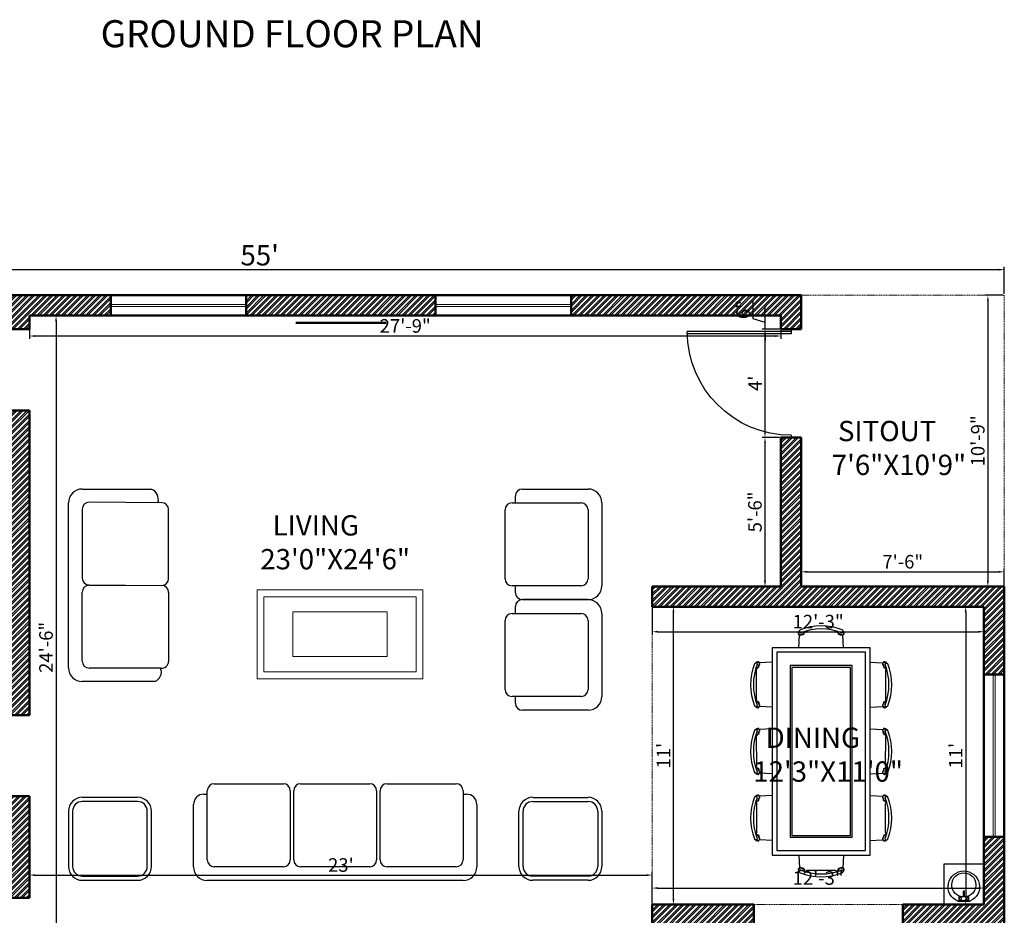
# Model space of a CAD drawing. Units: inches. Extents: x 3590 to 5167, y 65 to 1917.
# Tile 6 of 100: x 3869 to 4306, y 314 to 711. Entities that reach past the tile are written whole.
import ezdxf

# ---------------------------------------------------------------- set-up
doc = ezdxf.new("R2010")
doc.units = ezdxf.units.IN
doc.linetypes.add('DASHED', pattern=[0.75, 0.5, -0.25])
for name, color, linetype, lineweight in [('A-ANNO-DIMS', 2, 'Continuous', 18), ('A-ANNO-TEXT', 7, 'Continuous', 25), ('A-AREA-IDEN', 7, 'Continuous', 18), ('A-DOOR', 3, 'Continuous', 25), ('A-FLOR-FIXT', 8, 'Continuous', 18), ('A-FURN', 21, 'Continuous', 18), ('A-GLAZ', 4, 'Continuous', 18), ('A-WALL', 7, 'Continuous', 50), ('A-WALL-PATT', 251, 'Continuous', 13), ('S-BEAM-OVHD', 7, 'DASHED', 18)]:
    doc.layers.add(name, color=color, linetype=linetype, lineweight=lineweight)
for name, color, linetype in [('FUR', 42, 'Continuous'), ('HA', 9, 'Continuous'), ('M40-KOLTUKSUNGERI', 136, 'Continuous'), ('SANTEH', 7, 'Continuous'), ('wood', 26, 'Continuous')]:
    doc.layers.add(name, color=color, linetype=linetype)
doc.styles.get("Standard").update_dxf_attribs({"font": 'arial.ttf'})
doc.dimstyles.new('ISO-25', dxfattribs={"dimtxt": 9, "dimasz": 2.5, "dimexe": 1.25, "dimexo": 0.625, "dimtad": 1, "dimdec": 1, "dimlunit": 3, "dimtxsty": 'Standard', "dimcen": 2.5, "dimadec": 0, "dimazin": 0, "dimtfac": 1, "dimtdec": 1, "dimtmove": 0, "dimatfit": 3, "dimfxl": 1, "dimarcsym": 0})

# ---------------------------------------------------------------- blocks, each defined once
blk = doc.blocks.new('*D247')
at = {"layer": 'A-ANNO-DIMS', "color": 0, "lineweight": -2, "transparency": 16777216}
for p, q in [((3645.51, 589.68), (3645.51, 601.68)), ((3648.01, 600.43), (4303.01, 600.43)), ((4305.51, 589.68), (4305.51, 601.68))]:
    blk.add_line(p, q, dxfattribs=at)
at = {"layer": 'A-ANNO-DIMS', "color": 0, "transparency": 16777216}
for points in [[(3648.01, 600.84), (3648.01, 600.01), (3645.51, 600.43)], [(4303.01, 600.84), (4303.01, 600.01), (4305.51, 600.43)]]:
    blk.add_solid(points, dxfattribs=at)
at = {"layer": 'Defpoints', "color": 0, "transparency": 16777216}
for p in [(4305.51, 600.43), (3645.51, 589.06), (4305.51, 589.06)]:
    blk.add_point(p, dxfattribs=at)
at = {"layer": 'A-ANNO-DIMS', "color": 0, "transparency": 16777216, "insert": (3975.51, 605.63), "char_height": 9, "attachment_point": 5}
blk.add_mtext("55'", dxfattribs=at)
blk = doc.blocks.new('D')
for p, q in [((1, 0), (1, 46)), ((2, 0), (2, 46)), ((0, 0), (2, 0)), ((47, 0), (48, 0))]:
    blk.add_line(p, q)
at = {"ltscale": 0.5}
blk.add_arc((1, 0), 46, 0, 90, dxfattribs=at)
blk = doc.blocks.new('*D242')
at = {"layer": 'A-ANNO-DIMS', "color": 0, "lineweight": -2, "transparency": 16777216}
for p, q in [((4149.51, 450.43), (4149.51, 438.73)), ((4296.51, 450.43), (4296.51, 438.73)), ((4152.01, 439.98), (4294.01, 439.98))]:
    blk.add_line(p, q, dxfattribs=at)
at = {"layer": 'A-ANNO-DIMS', "color": 0, "transparency": 16777216}
for points in [[(4152.01, 440.4), (4152.01, 439.56), (4149.51, 439.98)], [(4294.01, 440.4), (4294.01, 439.56), (4296.51, 439.98)]]:
    blk.add_solid(points, dxfattribs=at)
at = {"layer": 'Defpoints', "color": 0, "transparency": 16777216}
for p in [(4149.51, 451.06), (4296.51, 451.06), (4296.51, 439.98)]:
    blk.add_point(p, dxfattribs=at)
at = {"layer": 'A-ANNO-DIMS', "color": 0, "transparency": 16777216, "insert": (4223.01, 443.67), "char_height": 6, "attachment_point": 5}
blk.add_mtext('12\'-3"', dxfattribs=at)
blk = doc.blocks.new('*D243')
at = {"layer": 'A-ANNO-DIMS', "color": 0, "lineweight": -2, "transparency": 16777216}
for p, q in [((4295.89, 451.06), (4287.14, 451.06)), ((4288.39, 448.56), (4288.39, 321.56)), ((4295.89, 319.06), (4287.14, 319.06))]:
    blk.add_line(p, q, dxfattribs=at)
at = {"layer": 'A-ANNO-DIMS', "color": 0, "transparency": 16777216}
for points in [[(4287.97, 448.56), (4288.81, 448.56), (4288.39, 451.06)], [(4287.97, 321.56), (4288.81, 321.56), (4288.39, 319.06)]]:
    blk.add_solid(points, dxfattribs=at)
at = {"layer": 'Defpoints', "color": 0, "transparency": 16777216}
for p in [(4296.51, 451.06), (4288.39, 319.06), (4296.51, 319.06)]:
    blk.add_point(p, dxfattribs=at)
at = {"layer": 'A-ANNO-DIMS', "color": 0, "transparency": 16777216, "insert": (4284.75, 385.06), "char_height": 6, "attachment_point": 5, "rotation": 90}
blk.add_mtext("11'", dxfattribs=at)
blk = doc.blocks.new('*D244')
at = {"layer": 'A-ANNO-DIMS', "color": 0, "lineweight": -2, "transparency": 16777216}
for p, q in [((4149.51, 319.68), (4149.51, 327.62)), ((4296.51, 319.68), (4296.51, 327.62)), ((4152.01, 326.37), (4294.01, 326.37))]:
    blk.add_line(p, q, dxfattribs=at)
at = {"layer": 'A-ANNO-DIMS', "color": 0, "transparency": 16777216}
for points in [[(4152.01, 326.79), (4152.01, 325.96), (4149.51, 326.37)], [(4294.01, 326.79), (4294.01, 325.96), (4296.51, 326.37)]]:
    blk.add_solid(points, dxfattribs=at)
at = {"layer": 'Defpoints', "color": 0, "transparency": 16777216}
for p in [(4296.51, 326.37), (4149.51, 319.06), (4296.51, 319.06)]:
    blk.add_point(p, dxfattribs=at)
at = {"layer": 'A-ANNO-DIMS', "color": 0, "transparency": 16777216, "insert": (4223.01, 330.06), "char_height": 6, "attachment_point": 5}
blk.add_mtext('12\'-3"', dxfattribs=at)
blk = doc.blocks.new('*D245')
at = {"layer": 'A-ANNO-DIMS', "color": 0, "lineweight": -2, "transparency": 16777216}
for p, q in [((4150.14, 451.06), (4160.13, 451.06)), ((4158.88, 321.56), (4158.88, 448.56)), ((4150.14, 319.06), (4160.13, 319.06))]:
    blk.add_line(p, q, dxfattribs=at)
at = {"layer": 'A-ANNO-DIMS', "color": 0, "transparency": 16777216}
for points in [[(4158.47, 448.56), (4159.3, 448.56), (4158.88, 451.06)], [(4158.47, 321.56), (4159.3, 321.56), (4158.88, 319.06)]]:
    blk.add_solid(points, dxfattribs=at)
at = {"layer": 'Defpoints', "color": 0, "transparency": 16777216}
for p in [(4149.51, 451.06), (4158.88, 451.06), (4149.51, 319.06)]:
    blk.add_point(p, dxfattribs=at)
at = {"layer": 'A-ANNO-DIMS', "color": 0, "transparency": 16777216, "insert": (4155.25, 385.06), "char_height": 6, "attachment_point": 5, "rotation": 90}
blk.add_mtext("11'", dxfattribs=at)
blk = doc.blocks.new('*D246')
at = {"layer": 'A-ANNO-DIMS', "color": 0, "lineweight": -2, "transparency": 16777216}
for p, q in [((4215.51, 460.68), (4215.51, 467.77)), ((4305.51, 460.68), (4305.51, 467.77)), ((4218.01, 466.52), (4303.01, 466.52))]:
    blk.add_line(p, q, dxfattribs=at)
at = {"layer": 'A-ANNO-DIMS', "color": 0, "transparency": 16777216}
for points in [[(4218.01, 466.93), (4218.01, 466.1), (4215.51, 466.52)], [(4303.01, 466.93), (4303.01, 466.1), (4305.51, 466.52)]]:
    blk.add_solid(points, dxfattribs=at)
at = {"layer": 'Defpoints', "color": 0, "transparency": 16777216}
for p in [(4305.51, 466.52), (4215.51, 460.06), (4305.51, 460.06)]:
    blk.add_point(p, dxfattribs=at)
at = {"layer": 'A-ANNO-DIMS', "color": 0, "transparency": 16777216, "insert": (4260.51, 470.21), "char_height": 6, "attachment_point": 5}
blk.add_mtext('7\'-6"', dxfattribs=at)
blk = doc.blocks.new('*D164')
at = {"layer": 'A-ANNO-DIMS', "color": 0, "lineweight": -2, "transparency": 16777216}
for p, q in [((4304.89, 589.06), (4296.98, 589.06)), ((4298.23, 586.56), (4298.23, 462.56)), ((4304.89, 460.06), (4296.98, 460.06))]:
    blk.add_line(p, q, dxfattribs=at)
at = {"layer": 'A-ANNO-DIMS', "color": 0, "transparency": 16777216}
for points in [[(4297.81, 586.56), (4298.64, 586.56), (4298.23, 589.06)], [(4297.81, 462.56), (4298.64, 462.56), (4298.23, 460.06)]]:
    blk.add_solid(points, dxfattribs=at)
at = {"layer": 'Defpoints', "color": 0, "transparency": 16777216}
for p in [(4305.51, 589.06), (4298.23, 460.06), (4305.51, 460.06)]:
    blk.add_point(p, dxfattribs=at)
at = {"layer": 'A-ANNO-DIMS', "color": 0, "transparency": 16777216, "insert": (4294.54, 524.56), "char_height": 6, "attachment_point": 5, "rotation": 90}
blk.add_mtext('10\'-9"', dxfattribs=at)
blk = doc.blocks.new('*D189')
at = {"layer": 'A-ANNO-DIMS', "color": 0, "lineweight": -2, "transparency": 16777216}
for p, q in [((3873.51, 579.43), (3873.51, 569.78)), ((4206.51, 579.43), (4206.51, 569.78)), ((3876.01, 571.03), (4204.01, 571.03))]:
    blk.add_line(p, q, dxfattribs=at)
at = {"layer": 'A-ANNO-DIMS', "color": 0, "transparency": 16777216}
for points in [[(3876.01, 571.44), (3876.01, 570.61), (3873.51, 571.03)], [(4204.01, 571.44), (4204.01, 570.61), (4206.51, 571.03)]]:
    blk.add_solid(points, dxfattribs=at)
at = {"layer": 'Defpoints', "color": 0, "transparency": 16777216}
for p in [(3873.51, 580.06), (4206.51, 580.06), (4206.51, 571.03)]:
    blk.add_point(p, dxfattribs=at)
at = {"layer": 'A-ANNO-DIMS', "color": 0, "transparency": 16777216, "insert": (4040.01, 574.72), "char_height": 6, "attachment_point": 5}
blk.add_mtext('27\'-9"', dxfattribs=at)
blk = doc.blocks.new('*D190')
at = {"layer": 'A-ANNO-DIMS', "color": 0, "lineweight": -2, "transparency": 16777216}
for p, q in [((4205.89, 526.06), (4198.22, 526.06)), ((4199.47, 462.56), (4199.47, 523.56)), ((4205.89, 460.06), (4198.22, 460.06))]:
    blk.add_line(p, q, dxfattribs=at)
at = {"layer": 'A-ANNO-DIMS', "color": 0, "transparency": 16777216}
for points in [[(4199.05, 523.56), (4199.89, 523.56), (4199.47, 526.06)], [(4199.05, 462.56), (4199.89, 462.56), (4199.47, 460.06)]]:
    blk.add_solid(points, dxfattribs=at)
at = {"layer": 'Defpoints', "color": 0, "transparency": 16777216}
for p in [(4199.47, 526.06), (4206.51, 526.06), (4206.51, 460.06)]:
    blk.add_point(p, dxfattribs=at)
at = {"layer": 'A-ANNO-DIMS', "color": 0, "transparency": 16777216, "insert": (4195.78, 493.06), "char_height": 6, "attachment_point": 5, "rotation": 90}
blk.add_mtext('5\'-6"', dxfattribs=at)
blk = doc.blocks.new('*D186')
at = {"layer": 'A-ANNO-DIMS', "color": 0, "lineweight": -2, "transparency": 16777216}
for p, q in [((4205.89, 574.06), (4198.22, 574.06)), ((4199.47, 528.56), (4199.47, 571.56)), ((4205.89, 526.06), (4198.22, 526.06))]:
    blk.add_line(p, q, dxfattribs=at)
at = {"layer": 'A-ANNO-DIMS', "color": 0, "transparency": 16777216}
for points in [[(4199.05, 571.56), (4199.89, 571.56), (4199.47, 574.06)], [(4199.05, 528.56), (4199.89, 528.56), (4199.47, 526.06)]]:
    blk.add_solid(points, dxfattribs=at)
at = {"layer": 'Defpoints', "color": 0, "transparency": 16777216}
for p in [(4199.47, 574.06), (4206.51, 574.06), (4206.51, 526.06)]:
    blk.add_point(p, dxfattribs=at)
at = {"layer": 'A-ANNO-DIMS', "color": 0, "transparency": 16777216, "insert": (4195.84, 550.06), "char_height": 6, "attachment_point": 5, "rotation": 90}
blk.add_mtext("4'", dxfattribs=at)
blk = doc.blocks.new('*D187')
at = {"layer": 'A-ANNO-DIMS', "color": 0, "lineweight": -2, "transparency": 16777216}
for p, q in [((4194.22, 578.64), (4194.22, 586.81)), ((4199.47, 582.56), (4199.47, 585.06)), ((4199.47, 577.06), (4194.22, 578.64)), ((4205.89, 580.06), (4198.22, 580.06)), ((4199.47, 574.06), (4199.47, 580.06)), ((4199.47, 574.06), (4199.47, 580.06)), ((4205.89, 574.06), (4198.22, 574.06)), ((4199.47, 571.56), (4199.47, 569.06))]:
    blk.add_line(p, q, dxfattribs=at)
at = {"layer": 'A-ANNO-DIMS', "color": 0, "transparency": 16777216}
for points in [[(4199.05, 582.56), (4199.89, 582.56), (4199.47, 580.06)], [(4199.05, 571.56), (4199.89, 571.56), (4199.47, 574.06)]]:
    blk.add_solid(points, dxfattribs=at)
at = {"layer": 'Defpoints', "color": 0, "transparency": 16777216}
for p in [(4199.47, 580.06), (4206.51, 580.06), (4206.51, 574.06)]:
    blk.add_point(p, dxfattribs=at)
at = {"layer": 'A-ANNO-DIMS', "color": 0, "transparency": 16777216, "insert": (4190.53, 582.72), "char_height": 6, "attachment_point": 5, "rotation": 90}
blk.add_mtext('6"', dxfattribs=at)
blk = doc.blocks.new('*D188')
at = {"layer": 'A-ANNO-DIMS', "color": 0, "lineweight": -2, "transparency": 16777216}
for p, q in [((3874.14, 580.06), (3886.54, 580.06)), ((3885.29, 577.56), (3885.29, 288.56)), ((3874.14, 286.06), (3886.54, 286.06))]:
    blk.add_line(p, q, dxfattribs=at)
at = {"layer": 'A-ANNO-DIMS', "color": 0, "transparency": 16777216}
for points in [[(3884.87, 577.56), (3885.7, 577.56), (3885.29, 580.06)], [(3884.87, 288.56), (3885.7, 288.56), (3885.29, 286.06)]]:
    blk.add_solid(points, dxfattribs=at)
at = {"layer": 'Defpoints', "color": 0, "transparency": 16777216}
for p in [(3873.51, 580.06), (3873.51, 286.06), (3885.29, 286.06)]:
    blk.add_point(p, dxfattribs=at)
at = {"layer": 'A-ANNO-DIMS', "color": 0, "transparency": 16777216, "insert": (3881.6, 433.06), "char_height": 6, "attachment_point": 5, "rotation": 90}
blk.add_mtext('24\'-6"', dxfattribs=at)
blk = doc.blocks.new('*D176')
at = {"layer": 'A-ANNO-DIMS', "color": 0, "lineweight": -2, "transparency": 16777216}
for p, q in [((3873.51, 322.68), (3873.51, 333.38)), ((3876.01, 332.13), (4147.01, 332.13)), ((4149.51, 319.68), (4149.51, 333.38))]:
    blk.add_line(p, q, dxfattribs=at)
at = {"layer": 'A-ANNO-DIMS', "color": 0, "transparency": 16777216}
for points in [[(3876.01, 332.55), (3876.01, 331.71), (3873.51, 332.13)], [(4147.01, 332.55), (4147.01, 331.71), (4149.51, 332.13)]]:
    blk.add_solid(points, dxfattribs=at)
at = {"layer": 'Defpoints', "color": 0, "transparency": 16777216}
for p in [(4149.51, 332.13), (3873.51, 322.06), (4149.51, 319.06)]:
    blk.add_point(p, dxfattribs=at)
at = {"layer": 'A-ANNO-DIMS', "color": 0, "transparency": 16777216, "insert": (4011.51, 335.82), "char_height": 6, "attachment_point": 5}
blk.add_mtext("23'", dxfattribs=at)
blk = doc.blocks.new('S1')
at = {"layer": 'M40-KOLTUKSUNGERI'}
for p, q in [((3.94, 27.4), (23.53, 27.4)), ((0, -23.47), (0, 23.47)), ((26.59, 23.52), (5.91, 23.65)), ((3.94, 21.68), (3.94, 2.06)), ((28.54, 1.93), (28.54, 21.55)), ((5.91, 0.09), (26.57, -0.04)), ((5.91, 0.03), (26.57, -0.04)), ((3.94, -21.63), (3.94, -1.94)), ((28.54, -1.94), (28.54, -21.67)), ((26.28, -23.6), (5.91, -23.6)), ((24.64, -27.4), (3.94, -27.4))]:
    blk.add_line(p, q, dxfattribs=at)
for centre, radius, start, end in [((3.94, 23.47), 3.94, 90, 180), ((22.44, 24.41), 3.19, 343.8468, 69.9238), ((5.91, 21.68), 1.97, 90, 180), ((26.57, 21.55), 1.97, 360, 90), ((5.91, 2.06), 1.97, 180, 270), ((5.91, -1.94), 1.97, 90, 180), ((26.57, 1.93), 1.97, 270, 0), ((26.57, -2.01), 1.97, 360, 90), ((5.91, -21.63), 1.97, 180, 270), ((26.6, -21.69), 1.94, 260.2828, 0.3826), ((3.94, -23.47), 3.94, 180, 270), ((23.58, -24.69), 2.91, 291.3314, 22.0931)]:
    blk.add_arc(centre, radius, start, end, dxfattribs=at)
blk = doc.blocks.new('S2')
at = {"layer": 'M40-KOLTUKSUNGERI'}
for p, q in [((-36.42, 5.91), (-36.42, 25.59)), ((-34.45, 27.56), (-14.76, 27.56)), ((-12.8, 25.59), (-12.8, 5.91)), ((-11.81, 5.91), (-11.81, 25.59)), ((-9.84, 27.56), (9.84, 27.56)), ((11.81, 25.59), (11.81, 5.91)), ((12.8, 5.91), (12.8, 25.59)), ((14.76, 27.56), (34.45, 27.56)), ((36.42, 25.59), (36.42, 5.91)), ((-37.4, 24.61), (-36.42, 24.61)), ((36.42, 24.61), (37.4, 24.61)), ((-40.35, 3.94), (-40.35, 21.65)), ((40.35, 21.65), (40.35, 3.94)), ((-14.76, 3.94), (-34.45, 3.94)), ((9.84, 3.94), (-9.84, 3.94)), ((34.45, 3.94), (14.76, 3.94)), ((36.42, 0), (-36.42, 0))]:
    blk.add_line(p, q, dxfattribs=at)
for centre, radius, start, end in [((-34.45, 25.59), 1.97, 90, 180), ((-14.76, 25.59), 1.97, 360, 90), ((-9.84, 25.59), 1.97, 90, 180), ((9.84, 25.59), 1.97, 360, 90), ((14.76, 25.59), 1.97, 90, 180), ((34.45, 25.59), 1.97, 360, 90), ((-37.4, 21.65), 2.95, 90, 180), ((37.4, 21.65), 2.95, 360, 90), ((-34.45, 5.91), 1.97, 180, 270), ((-14.76, 5.91), 1.97, 270, 0), ((-9.84, 5.91), 1.97, 180, 270), ((9.84, 5.91), 1.97, 270, 0), ((14.76, 5.91), 1.97, 180, 270), ((34.45, 5.91), 1.97, 270, 0), ((-36.42, 3.94), 3.94, 180, 270), ((36.42, 3.94), 3.94, 270, 0)]:
    blk.add_arc(centre, radius, start, end, dxfattribs=at)
blk = doc.blocks.new('S3')
at = {"layer": 'M40-KOLTUKSUNGERI'}
for p, q in [((-22.64, 15.75), (-3.94, 15.75)), ((-25.59, 11.81), (-5.91, 11.81)), ((-24.61, 11.81), (-24.61, 13.78)), ((0, 11.81), (0, -11.81)), ((-27.56, -9.84), (-27.56, 9.84)), ((-3.94, 9.84), (-3.94, -9.84)), ((-5.91, -11.81), (-25.59, -11.81)), ((-24.61, -13.78), (-24.61, -11.81)), ((-3.94, -15.75), (-22.64, -15.75))]:
    blk.add_line(p, q, dxfattribs=at)
for centre, radius, start, end in [((-22.64, 13.78), 1.97, 90, 180), ((-3.94, 11.81), 3.94, 360, 90), ((-25.59, 9.84), 1.97, 90, 180), ((-5.91, 9.84), 1.97, 360, 90), ((-25.59, -9.84), 1.97, 180, 270), ((-5.91, -9.84), 1.97, 270, 0), ((-22.64, -13.78), 1.97, 180, 270), ((-3.94, -11.81), 3.94, 270, 0)]:
    blk.add_arc(centre, radius, start, end, dxfattribs=at)
blk = doc.blocks.new('T1')
at = {"layer": 'M40-KOLTUKSUNGERI'}
for p, q in [((4762.34, 1687.13), (4746.59, 1687.13)), ((4762.34, 1685.95), (4746.59, 1685.95)), ((4742.65, 1683.2), (4742.65, 1667.45)), ((4743.83, 1683.2), (4743.83, 1667.45)), ((4765.09, 1667.45), (4765.09, 1683.2)), ((4766.27, 1667.45), (4766.27, 1683.2)), ((4746.59, 1664.69), (4762.34, 1664.69)), ((4746.59, 1663.51), (4762.34, 1663.51))]:
    blk.add_line(p, q, dxfattribs=at)
for centre, radius, start, end in [((4746.59, 1683.2), 3.94, 90, 180), ((4746.59, 1683.2), 2.76, 90, 180), ((4762.34, 1683.2), 3.94, 360, 90), ((4762.34, 1683.2), 2.76, 360, 90), ((4746.59, 1667.45), 3.94, 180, 270), ((4746.59, 1667.45), 2.76, 180, 270), ((4762.34, 1667.45), 3.94, 270, 0), ((4762.34, 1667.45), 2.76, 270, 0)]:
    blk.add_arc(centre, radius, start, end, dxfattribs=at)
blk = doc.blocks.new('T2')
at = {"layer": 'M40-KOLTUKSUNGERI'}
for p, q in [((4874.89, 1687.13), (4890.64, 1687.13)), ((4874.89, 1685.95), (4890.64, 1685.95)), ((4870.95, 1667.45), (4870.95, 1683.2)), ((4872.13, 1667.45), (4872.13, 1683.2)), ((4893.39, 1683.2), (4893.39, 1667.45)), ((4894.57, 1683.2), (4894.57, 1667.45)), ((4890.64, 1664.69), (4874.89, 1664.69)), ((4890.64, 1663.51), (4874.89, 1663.51))]:
    blk.add_line(p, q, dxfattribs=at)
for centre, radius, start, end in [((4874.89, 1683.2), 3.94, 90, 180), ((4874.89, 1683.2), 2.76, 90, 180), ((4890.64, 1683.2), 3.94, 360, 90), ((4890.64, 1683.2), 2.76, 360, 90), ((4874.89, 1667.45), 3.94, 180, 270), ((4874.89, 1667.45), 2.76, 180, 270), ((4890.64, 1667.45), 3.94, 270, 0), ((4890.64, 1667.45), 2.76, 270, 0)]:
    blk.add_arc(centre, radius, start, end, dxfattribs=at)
blk = doc.blocks.new('A$C39F63D19')
at = {"layer": 'FUR'}
for p, q in [((1.415, 2.447), (1.406, 2.455)), ((1.36, 2.386), (1.131, 2.157)), ((1.36, 2.402), (1.359, 2.403)), ((1.549, 2.326), (1.441, 2.424)), ((1.874, 2.232), (1.982, 2.329)), ((2.008, 2.352), (2.017, 2.36)), ((2.063, 2.307), (2.064, 2.308)), ((2.063, 2.292), (2.292, 2.063)), ((1.07, 2.102), (1.063, 2.111)), ((1.116, 2.157), (1.114, 2.158)), ((1.116, 2.157), (1.114, 2.158)), ((1.191, 1.969), (1.094, 2.076)), ((2.307, 2.063), (2.308, 2.064)), ((2.307, 2.063), (2.308, 2.064)), ((2.352, 2.008), (2.36, 2.017)), ((0.885, 1.916), (0.876, 1.924)), ((1.018, 1.796), (0.91, 1.893)), ((2.232, 1.874), (2.329, 1.982)), ((0.83, 1.856), (0.6, 1.627)), ((0.83, 1.871), (0.828, 1.873)), ((0.54, 1.572), (0.532, 1.581)), ((0.585, 1.627), (0.584, 1.628)), ((0.585, 1.627), (0.584, 1.628)), ((0.66, 1.438), (0.563, 1.546)), ((2.326, 1.549), (2.424, 1.441)), ((0.299, 1.341), (0.298, 1.342)), ((0.354, 1.386), (0.345, 1.394)), ((0.488, 1.266), (0.38, 1.363)), ((2.386, 1.36), (2.157, 1.131)), ((2.402, 1.36), (2.403, 1.359)), ((2.447, 1.415), (2.455, 1.406)), ((0.299, 1.326), (0.07, 1.097)), ((1.969, 1.191), (2.076, 1.094)), ((2.157, 1.116), (2.158, 1.114)), ((2.157, 1.116), (2.158, 1.114)), ((0.01, 1.042), (0.002, 1.05)), ((0.13, 0.908), (0.033, 1.016)), ((0.055, 1.097), (0.054, 1.098)), ((0.055, 1.097), (0.054, 1.098)), ((1.796, 1.018), (1.893, 0.91)), ((2.102, 1.07), (2.111, 1.063)), ((1.856, 0.83), (1.627, 0.6)), ((1.871, 0.83), (1.873, 0.828)), ((1.916, 0.885), (1.924, 0.876)), ((0.225, 0.583), (0.128, 0.475)), ((1.438, 0.66), (1.546, 0.563)), ((1.627, 0.585), (1.628, 0.584)), ((1.627, 0.585), (1.628, 0.584)), ((0.104, 0.449), (0.096, 0.44)), ((1.266, 0.488), (1.363, 0.38)), ((1.572, 0.54), (1.581, 0.532)), ((0.149, 0.394), (0.148, 0.393)), ((0.165, 0.394), (0.394, 0.165)), ((1.386, 0.354), (1.394, 0.345)), ((0.583, 0.225), (0.475, 0.128)), ((1.326, 0.299), (1.097, 0.07)), ((1.341, 0.299), (1.342, 0.298)), ((0.394, 0.149), (0.393, 0.148)), ((0.394, 0.149), (0.393, 0.148)), ((0.908, 0.13), (1.016, 0.033)), ((0.449, 0.104), (0.44, 0.096)), ((1.042, 0.01), (1.05, 0.002)), ((1.097, 0.055), (1.098, 0.054)), ((1.097, 0.055), (1.098, 0.054))]:
    blk.add_line(p, q, dxfattribs=at)
for points in [[(1.664, 2.442), (0.015, 0.793), (0.793, 0.015), (2.442, 1.664)], [(1.664, 2.371), (0.085, 0.793), (0.793, 0.085), (2.371, 1.664)], [(1.664, 2.159), (0.298, 0.793), (0.793, 0.298), (2.159, 1.664)]]:
    blk.add_lwpolyline(points, close=True, dxfattribs=at)
for centre, radius, start, end in [((1.657, 1.86), 0.652, 113.773, 156.227), ((1.399, 2.447), 0.0108, 48, 113.773), ((1.419, 2.446), 0.0101, 329.621, 147.4253), ((1.408, 2.439), 0.0108, 293.3306, 48), ((1.435, 2.438), 0.00795, 264.7688, 163.6538), ((1.657, 1.86), 0.62, 113.3306, 156.6694), ((1.352, 2.394), 0.0108, 315, 45), ((1.381, 2.407), 0.0085, 151.0497, 5.8544), ((1.399, 2.404), 0.0102, 161.256, 35.9951), ((1.416, 2.411), 0.00785, 184.4301, 31.8132), ((1.431, 2.421), 0.0103, 213.3009, 71.363), ((1.988, 2.344), 0.00795, 16.3462, 275.2312), ((1.992, 2.326), 0.0103, 108.637, 326.6991), ((2.004, 2.351), 0.0101, 32.5747, 210.379), ((2.015, 2.344), 0.0108, 132, 246.6694), ((1.765, 1.765), 0.62, 23.3306, 66.6694), ((2.024, 2.352), 0.0108, 66.227, 132), ((1.765, 1.765), 0.652, 23.773, 66.227), ((2.007, 2.316), 0.00785, 148.1868, 355.5699), ((2.023, 2.31), 0.0102, 144.0049, 18.744), ((2.041, 2.312), 0.0085, 174.1456, 28.9503), ((2.07, 2.3), 0.0108, 135, 225), ((1.071, 2.118), 0.0108, 156.227, 222), ((1.071, 2.099), 0.0101, 122.5747, 300.379), ((1.106, 2.102), 0.00785, 238.1868, 85.5699), ((1.11, 2.136), 0.0085, 264.1456, 118.9503), ((1.123, 2.165), 0.0108, 225, 315), ((1.078, 2.11), 0.0108, 222, 336.6694), ((1.079, 2.082), 0.00795, 106.3462, 5.2312), ((1.096, 2.086), 0.0103, 198.637, 56.6991), ((2.3, 2.07), 0.0108, 225, 315), ((2.31, 2.023), 0.0102, 71.256, 305.9951), ((2.312, 2.041), 0.0085, 61.0497, 275.8544), ((2.316, 2.007), 0.00785, 94.4301, 301.8132), ((2.326, 1.992), 0.0103, 123.3009, 341.363), ((2.344, 2.015), 0.0108, 203.3306, 318), ((2.344, 1.988), 0.00795, 174.7688, 73.6538), ((2.351, 2.004), 0.0101, 239.621, 57.4253), ((2.352, 2.024), 0.0108, 318, 23.773), ((1.127, 1.33), 0.652, 113.773, 156.227), ((1.127, 1.33), 0.62, 113.3306, 156.6694), ((0.869, 1.916), 0.0108, 48, 113.773), ((0.885, 1.881), 0.00785, 184.4301, 31.8132), ((0.888, 1.915), 0.0101, 329.621, 147.4253), ((0.877, 1.908), 0.0108, 293.3306, 48), ((0.901, 1.89), 0.0103, 213.3009, 71.363), ((0.905, 1.908), 0.00795, 264.7688, 163.6538), ((0.822, 1.864), 0.0108, 315, 45), ((0.851, 1.876), 0.0085, 151.0497, 5.8544), ((0.869, 1.874), 0.0102, 161.256, 35.9951), ((0.54, 1.588), 0.0108, 156.227, 222), ((0.541, 1.568), 0.0101, 122.5747, 300.379), ((0.548, 1.579), 0.0108, 222, 336.6694), ((0.548, 1.552), 0.00795, 106.3462, 5.2312), ((0.566, 1.556), 0.0103, 198.637, 56.6991), ((0.576, 1.571), 0.00785, 238.1868, 85.5699), ((0.58, 1.606), 0.0085, 264.1456, 118.9503), ((0.583, 1.587), 0.0102, 234.0049, 108.744), ((0.593, 1.635), 0.0108, 225, 315), ((2.421, 1.431), 0.0103, 18.637, 236.6991), ((2.438, 1.435), 0.00795, 286.3462, 185.2312), ((0.597, 0.799), 0.652, 113.773, 156.227), ((0.597, 0.799), 0.62, 113.3306, 156.6694), ((0.292, 1.333), 0.0108, 315, 45), ((0.321, 1.346), 0.0085, 151.0497, 5.8544), ((0.339, 1.344), 0.0102, 161.256, 35.9951), ((0.338, 1.386), 0.0108, 48, 113.773), ((0.355, 1.35), 0.00785, 184.4301, 31.8132), ((0.358, 1.385), 0.0101, 329.621, 147.4253), ((0.347, 1.378), 0.0108, 293.3306, 48), ((0.37, 1.36), 0.0103, 213.3009, 71.363), ((0.374, 1.378), 0.00795, 264.7688, 163.6538), ((1.86, 1.657), 0.62, 293.3306, 336.6694), ((1.86, 1.657), 0.652, 293.773, 336.227), ((2.394, 1.352), 0.0108, 45, 135), ((2.404, 1.399), 0.0102, 54.0049, 288.744), ((2.407, 1.381), 0.0085, 84.1456, 298.9503), ((2.411, 1.416), 0.00785, 58.1868, 265.5699), ((2.439, 1.408), 0.0108, 42, 156.6694), ((2.446, 1.419), 0.0101, 302.5747, 120.379), ((2.447, 1.399), 0.0108, 336.227, 42), ((2.102, 1.106), 0.00785, 4.4301, 211.8132), ((2.118, 1.113), 0.0102, 341.256, 215.9951), ((2.136, 1.11), 0.0085, 331.0497, 185.8544), ((2.165, 1.123), 0.0108, 135, 225), ((0.01, 1.058), 0.0108, 156.227, 222), ((0.011, 1.038), 0.0101, 122.5747, 300.379), ((0.018, 1.049), 0.0108, 222, 336.6694), ((0.018, 1.022), 0.00795, 106.3462, 5.2312), ((0.036, 1.026), 0.0103, 198.637, 56.6991), ((0.046, 1.041), 0.00785, 238.1868, 85.5699), ((0.05, 1.075), 0.0085, 264.1456, 118.9503), ((0.052, 1.057), 0.0102, 234.0049, 108.744), ((0.063, 1.104), 0.0108, 225, 315), ((2.082, 1.079), 0.00795, 84.7688, 343.6538), ((2.086, 1.096), 0.0103, 33.3009, 251.363), ((2.099, 1.071), 0.0101, 149.621, 327.4253), ((2.11, 1.078), 0.0108, 113.3306, 228), ((2.118, 1.071), 0.0108, 228, 293.773), ((1.881, 0.885), 0.00785, 58.1868, 265.5699), ((1.89, 0.901), 0.0103, 18.637, 236.6991), ((1.908, 0.877), 0.0108, 42, 156.6694), ((1.908, 0.905), 0.00795, 286.3462, 185.2312), ((1.915, 0.888), 0.0101, 302.5747, 120.379), ((1.33, 1.127), 0.62, 293.3306, 336.6694), ((1.33, 1.127), 0.652, 293.773, 336.227), ((1.864, 0.822), 0.0108, 45, 135), ((1.874, 0.869), 0.0102, 54.0049, 288.744), ((1.876, 0.851), 0.0085, 84.1456, 298.9503), ((1.916, 0.869), 0.0108, 336.227, 42), ((1.552, 0.548), 0.00795, 84.7688, 343.6538), ((1.556, 0.566), 0.0103, 33.3009, 251.363), ((1.571, 0.576), 0.00785, 4.4301, 211.8132), ((1.579, 0.548), 0.0108, 113.3306, 228), ((1.587, 0.583), 0.0102, 341.256, 215.9951), ((1.606, 0.58), 0.0085, 331.0497, 185.8544), ((1.635, 0.593), 0.0108, 135, 225), ((0.105, 0.452), 0.0101, 59.621, 237.4253), ((0.112, 0.442), 0.0108, 23.3306, 138), ((0.113, 0.469), 0.00795, 354.7688, 253.6538), ((0.13, 0.465), 0.0103, 303.3009, 161.363), ((0.691, 0.691), 0.62, 203.3306, 246.6694), ((0.14, 0.449), 0.00785, 274.4301, 121.8132), ((0.147, 0.433), 0.0102, 251.256, 125.9951), ((1.568, 0.541), 0.0101, 149.621, 327.4253), ((1.588, 0.54), 0.0108, 228, 293.773), ((0.104, 0.433), 0.0108, 138, 203.773), ((0.691, 0.691), 0.652, 203.773, 246.227), ((0.144, 0.415), 0.0085, 241.0497, 95.8544), ((0.157, 0.386), 0.0108, 45, 135), ((0.799, 0.597), 0.62, 293.3306, 336.6694), ((0.799, 0.597), 0.652, 293.773, 336.227), ((1.344, 0.339), 0.0102, 54.0049, 288.744), ((1.35, 0.355), 0.00785, 58.1868, 265.5699), ((1.36, 0.37), 0.0103, 18.637, 236.6991), ((1.378, 0.347), 0.0108, 42, 156.6694), ((1.378, 0.374), 0.00795, 286.3462, 185.2312), ((1.385, 0.358), 0.0101, 302.5747, 120.379), ((1.386, 0.338), 0.0108, 336.227, 42), ((1.333, 0.292), 0.0108, 45, 135), ((1.346, 0.321), 0.0085, 84.1456, 298.9503), ((0.386, 0.157), 0.0108, 315, 45), ((0.415, 0.144), 0.0085, 354.1456, 208.9503), ((0.433, 0.147), 0.0102, 324.0049, 198.744), ((0.449, 0.14), 0.00785, 328.1868, 175.5699), ((0.442, 0.112), 0.0108, 312, 66.6694), ((0.465, 0.13), 0.0103, 288.637, 146.6991), ((0.469, 0.113), 0.00795, 196.3462, 95.2312), ((0.433, 0.104), 0.0108, 246.227, 312), ((0.452, 0.105), 0.0101, 212.5747, 30.379), ((1.022, 0.018), 0.00795, 84.7688, 343.6538), ((1.026, 0.036), 0.0103, 33.3009, 251.363), ((1.038, 0.011), 0.0101, 149.621, 327.4253), ((1.041, 0.046), 0.00785, 4.4301, 211.8132), ((1.049, 0.018), 0.0108, 113.3306, 228), ((1.057, 0.052), 0.0102, 341.256, 215.9951), ((1.058, 0.01), 0.0108, 228, 293.773), ((1.075, 0.05), 0.0085, 331.0497, 185.8544), ((1.104, 0.063), 0.0108, 135, 225)]:
    blk.add_arc(centre, radius, start, end, dxfattribs=at)
at = {"layer": 'HA'}
blk.add_lwpolyline([(1.664, 2.131), (0.326, 0.793), (0.793, 0.326), (2.131, 1.664)], close=True, dxfattribs=at)
at = {"layer": 'wood'}
for points in [[(1.383, 2.415, 0.308332), (1.374, 2.411, -0.00386)], [(1.41, 2.406, -0.15729), (1.408, 2.41, -0.120016)], [(1.111, 2.108, 1.044756), (1.114, 2.128, -0.117685), (1.11, 2.127, -1.643727), (1.107, 2.11, -0.15729)], [(2.316, 2.015, -0.120016), (2.311, 2.013, -0.15729)], [(0.852, 1.885, 0.308332), (0.844, 1.881, -0.00386)], [(0.879, 1.876, -0.15729), (0.877, 1.88, -0.120016)], [(0.581, 1.577, 1.044756), (0.583, 1.598, -0.117685), (0.579, 1.597, -1.643727), (0.577, 1.579, -0.15729)], [(0.349, 1.345, -0.15729), (0.347, 1.35, -0.120016)], [(2.41, 1.408, -0.15729), (2.406, 1.41, 1.044756), (2.404, 1.389, -0.117685), (2.408, 1.39, -1.643727)], [(2.11, 1.107, -0.120016), (2.108, 1.111, -0.15729)], [(2.135, 1.102, 0.308332), (2.143, 1.106, -0.00386)], [(1.88, 0.877, -0.15729), (1.876, 0.879, 1.044756), (1.873, 0.859, -0.117685), (1.877, 0.86, -1.643727)], [(1.579, 0.577, -0.120016), (1.577, 0.581, -0.15729)], [(1.604, 0.572, 0.308332), (1.613, 0.576, -0.00386)], [(0.145, 0.443, -0.15729), (0.141, 0.442, -0.120016)], [(1.35, 0.347, -0.15729), (1.345, 0.349, 1.044756), (1.343, 0.329, -0.117685), (1.347, 0.329, -1.643727)], [(1.049, 0.046, -0.120016), (1.047, 0.051, -0.15729)], [(1.074, 0.041, 0.308332), (1.083, 0.046, -0.00386)]]:
    blk.add_lwpolyline(points, format="xyb", close=True, dxfattribs=at)
blk = doc.blocks.new('r11')
at = {"layer": 'SANTEH', "ltscale": 5}
for p, q in [((0, 0), (600, 0)), ((0, -600), (0, 0)), ((600, 0), (600, -600)), ((210, -50), (390, -50)), ((210, -50), (210, -50)), ((224, -63), (376, -63)), ((224, -113), (224, -63)), ((376, -113), (224, -113)), ((233, -79), (249, -69)), ((233, -98), (233, -79)), ((249, -107), (233, -98)), ((249, -69), (266, -79)), ((266, -98), (249, -107)), ((266, -79), (266, -98)), ((288, -202), (288, -113)), ((312, -113), (312, -202)), ((334, -79), (351, -69)), ((334, -98), (334, -79)), ((351, -107), (334, -98)), ((351, -69), (367, -79)), ((367, -98), (351, -107)), ((367, -79), (367, -98)), ((376, -63), (376, -113)), ((312, -184), (288, -184)), ((312, -202), (288, -202)), ((600, -600), (0, -600))]:
    blk.add_line(p, q, dxfattribs=at)
for centre, radius, start, end in [((300, -266), 234, 112.5, 67.5), ((300, -293), 180, 93.8183, 86.1817)]:
    blk.add_arc(centre, radius, start, end, dxfattribs=at)

msp = doc.modelspace()

# ---------------------------------------------------------------- hatches: boundary and pattern name
at = {"layer": 'A-WALL-PATT', "transparency": 33554687}
h = msp.add_hatch(dxfattribs=at)
h.set_pattern_fill('ANSI32', color=256, scale=0.2)
h.set_pattern_definition([(45, (0, -1216.9392), (-1.3470384, 1.3470384), []), (45, (0.898, -1216.9392), (-1.3470384, 1.3470384), [])])
h.paths.add_polyline_path([(3768.51, 589.06), (3645.51, 589.06), (3645.51, 568.06), (3654.51, 568.06), (3654.51, 580.06), (3671.16, 580.06), (3768.51, 580.06)])
h.paths.add_polyline_path([(3909.51, 589.06), (3816.51, 589.06), (3816.51, 580.06), (3864.51, 580.06), (3864.51, 574.06), (3873.51, 574.06), (3873.51, 580.06), (3909.51, 580.06)])
h.paths.add_polyline_path([(4053.51, 589.06), (3969.51, 589.06), (3969.51, 580.06), (4053.51, 580.06)])
h.paths.add_polyline_path([(4215.51, 589.06), (4113.51, 589.06), (4113.51, 580.06), (4206.51, 580.06), (4206.51, 574.06), (4215.51, 574.06)])
h.paths.add_polyline_path([(3654.51, 520.06), (3645.51, 520.06), (3645.51, 403.06), (3654.51, 403.06), (3654.51, 433.06), (3741.51, 433.06), (3741.51, 439.06), (3654.51, 439.06)], flags=17)
h.paths.add_polyline_path([(3873.51, 538.06), (3864.51, 538.06), (3864.51, 439.06), (3771.51, 439.06), (3771.51, 433.06), (3774.51, 433.06), (3774.51, 337.06), (3654.51, 337.06), (3654.51, 367.06), (3645.51, 367.06), (3645.51, 322.06), (3654.51, 322.06), (3654.51, 328.06), (3864.51, 328.06), (3864.51, 322.06), (3873.51, 322.06), (3873.51, 367.06), (3864.51, 367.06), (3864.51, 337.06), (3780.51, 337.06), (3780.51, 433.06), (3864.51, 433.06), (3864.51, 403.06), (3873.51, 403.06)])
h.paths.add_polyline_path([(3654.51, 274.06), (3645.51, 274.06), (3645.51, 109.06), (3810.51, 109.06), (3810.51, 118.06), (3809.96, 118.06), (3654.51, 118.06)])
h.paths.add_polyline_path([(3915.51, 118.06), (3873.51, 118.06), (3873.51, 135.93), (3873.51, 205.06), (3876.51, 205.06), (3876.51, 214.06), (3864.51, 214.06), (3864.51, 118.06), (3858.51, 118.06), (3858.51, 109.06), (3915.51, 109.06)])
h.paths.add_polyline_path([(4028.01, 118.06), (4002.51, 118.06), (4002.51, 286.06), (3981.51, 286.06), (3981.51, 277.06), (3993.51, 277.06), (3993.51, 214.06), (3921.51, 214.06), (3921.51, 277.06), (3933.51, 277.06), (3933.51, 286.06), (3864.51, 286.06), (3864.51, 277.06), (3912.51, 277.06), (3912.51, 214.06), (3906.51, 214.06), (3906.51, 205.06), (3993.51, 205.06), (3993.51, 118.06), (3951.51, 118.06), (3951.51, 109.06), (4028.01, 109.06)])
h.paths.add_polyline_path([(4203.51, 118.06), (4158.51, 118.06), (4158.51, 310.06), (4194.51, 310.06), (4194.51, 319.06), (4149.51, 319.06), (4149.51, 118.06), (4124.01, 118.06), (4124.01, 109.06), (4203.51, 109.06)])
h.paths.add_polyline_path([(4305.51, 349.06), (4296.51, 349.06), (4296.51, 319.06), (4278.64, 319.06), (4260.51, 319.06), (4260.51, 310.06), (4296.51, 310.06), (4296.51, 304.06), (4305.51, 304.06)])
h.paths.add_polyline_path([(4305.51, 256.06), (4296.51, 256.06), (4296.51, 118.06), (4251.51, 118.06), (4251.51, 109.06), (4305.51, 109.06)])
h.paths.add_polyline_path([(4305.51, 460.06), (4215.51, 460.06), (4215.51, 526.06), (4206.51, 526.06), (4206.51, 460.06), (4149.51, 460.06), (4149.51, 451.06), (4296.51, 451.06), (4296.51, 421.06), (4305.51, 421.06)])

# ---------------------------------------------------------------- linework, layer by layer
at = {"layer": 'A-FURN'}
for points in [[(3974.36, 458.56), (4047.86, 458.56), (4047.86, 419.13), (3974.36, 419.13)], [(3977.42, 455.49), (4044.8, 455.49), (4044.8, 422.19), (3977.42, 422.19)], [(3990.24, 448.76), (4031.98, 448.76), (4031.98, 428.93), (3990.24, 428.93)]]:
    msp.add_lwpolyline(points, close=True, dxfattribs=at)
at = {"layer": 'A-GLAZ'}
for p, q in [((3969.51, 585.06), (3909.51, 585.06)), ((4113.51, 585.06), (4053.51, 585.06)), ((3969.51, 584.06), (3909.51, 584.06)), ((4113.51, 584.06), (4053.51, 584.06)), ((4300.51, 349.06), (4300.51, 421.06)), ((4301.51, 349.06), (4301.51, 421.06))]:
    msp.add_line(p, q, dxfattribs=at)
at = {"layer": 'A-WALL'}
for p, q in [((3909.51, 580.06), (3909.51, 589.06)), ((3969.51, 580.06), (3969.51, 589.06)), ((4053.51, 580.06), (4053.51, 589.06)), ((4113.51, 580.06), (4113.51, 589.06)), ((4215.51, 589.06), (4215.51, 574.06)), ((3873.51, 580.06), (4206.51, 580.06)), ((3873.51, 574.06), (3873.51, 580.06)), ((3991.51, 576.87), (4031.51, 576.87)), ((4206.51, 580.06), (4206.51, 574.06)), ((3864.51, 574.06), (3873.51, 574.06)), ((4206.51, 574.06), (4215.51, 574.06)), ((3864.51, 538.06), (3873.51, 538.06)), ((3873.51, 403.06), (3873.51, 538.06)), ((4206.51, 526.06), (4206.51, 460.06)), ((4206.51, 526.06), (4215.51, 526.06)), ((4215.51, 526.06), (4215.51, 460.06)), ((4206.51, 460.06), (4149.51, 460.06)), ((4149.51, 451.06), (4149.51, 460.06)), ((4305.51, 460.06), (4215.51, 460.06)), ((4296.51, 451.06), (4149.51, 451.06)), ((4296.51, 451.06), (4296.51, 319.06)), ((4296.51, 421.06), (4305.51, 421.06)), ((3864.51, 403.06), (3873.51, 403.06)), ((3864.51, 367.06), (3873.51, 367.06)), ((3873.51, 322.06), (3873.51, 367.06)), ((4296.51, 349.06), (4305.51, 349.06)), ((3873.51, 322.06), (3864.51, 322.06)), ((4194.51, 319.06), (4149.51, 319.06)), ((4149.51, 118.06), (4149.51, 319.06)), ((4194.51, 310.06), (4194.51, 319.06)), ((4296.51, 319.06), (4260.51, 319.06)), ((4260.51, 310.06), (4260.51, 319.06))]:
    msp.add_line(p, q, dxfattribs=at)
msp.add_lwpolyline([(4305.51, 460.06), (4305.51, 109.06), (3645.51, 109.06), (3645.51, 589.06), (4215.51, 589.06)], dxfattribs=at)
at = {"layer": 'S-BEAM-OVHD'}
for p, q in [((4215.51, 589.06), (4305.51, 589.06)), ((4305.51, 589.06), (4305.51, 460.06)), ((4149.51, 451.06), (4149.51, 319.06)), ((4194.51, 319.06), (4260.51, 319.06))]:
    msp.add_line(p, q, dxfattribs=at)

# ---------------------------------------------------------------- block references
at = {"layer": 'A-DOOR', "xscale": -1, "rotation": 90}
msp.add_blockref('D', (4211.01, 574.06), dxfattribs=at)
at = {"layer": 'A-FLOR-FIXT', "xscale": -0.0297800069284724, "yscale": 0.0297800069284724, "zscale": 0.0297800069284724, "rotation": 180}
msp.add_blockref('r11', (4278.64, 319.06), dxfattribs=at)
at = {"layer": 'A-FURN', "xscale": 1.555868517605225, "yscale": 1.555868517605225, "zscale": 1.555868517605225}
for name, p in [('S1', (3890.75, 460.56)), ('S3', (4127.16, 478.7)), ('S3', (4127.16, 429.69)), ('S2', (4008.98, 329.71)), ('T1', (-3488.15, -2258.38)), ('T2', (-3488.15, -2258.38))]:
    msp.add_blockref(name, p, dxfattribs=at)
at = {"layer": 'A-FURN', "xscale": 39.3701, "yscale": 39.3701, "zscale": 39.3701, "rotation": 225.0000000000003}
msp.add_blockref('A$C39F63D19', (4224.35, 455.33), dxfattribs=at)

# ---------------------------------------------------------------- texts
at = {"layer": 'A-ANNO-TEXT', "insert": (3905.03, 710.99), "char_height": 12, "attachment_point": 1}
msp.add_mtext_dynamic_manual_height_columns('{\\fTimes New Roman|b0|i0|c0|p18;GROUND FLOOR PLAN}', width=197.6934, gutter_width=12.5, heights=[0], dxfattribs=at)
at = {"layer": 'A-AREA-IDEN', "char_height": 9, "attachment_point": 1}
for s, insert in [('{\\fTimes New Roman|b0|i0|c0|p18; SITOUT\\P7\'6"X10\'9"}', (4229.04, 533.42)), ('{\\fTimes New Roman|b0|i0|c0|p18;  LIVING\\P23\'0"X24\'6"}', (3975.77, 491.62)), ('{\\fTimes New Roman|b0|i0|c0|p18;  DINING\\P12\'3"X11\'0"}', (4194.24, 397.51))]:
    msp.add_mtext_dynamic_manual_height_columns(s, width=67.3508, gutter_width=12.5, heights=[0], dxfattribs=dict(at, insert=insert))

# ---------------------------------------------------------------- dimensions: what is measured, and where the dimension line sits
at = {"layer": 'A-ANNO-DIMS'}
for base, p1, p2, override, picture, middle in [((4305.51, 600.43), (3645.51, 589.06), (4305.51, 589.06), {"dimclrd": 0, "dimclre": 0, "dimclrt": 0}, '*D247', (3975.51, 605.63)), ((4206.51, 571.03), (3873.51, 580.06), (4206.51, 580.06), {"dimtxt": 6, "dimclrd": 0, "dimclre": 0, "dimclrt": 0}, '*D189', (4040.01, 574.72)), ((4305.51, 466.52), (4215.51, 460.06), (4305.51, 460.06), {"dimtxt": 6, "dimclrd": 0, "dimclre": 0, "dimclrt": 0}, '*D246', (4260.51, 470.21)), ((4296.51, 439.98), (4149.51, 451.06), (4296.51, 451.06), {"dimtxt": 6, "dimclrd": 0, "dimclre": 0, "dimclrt": 0}, '*D242', (4223.01, 443.67)), ((4149.51, 332.13), (3873.51, 322.06), (4149.51, 319.06), {"dimtxt": 6, "dimclrd": 0, "dimclre": 0, "dimclrt": 0}, '*D176', (4011.51, 335.82)), ((4296.51, 326.37), (4149.51, 319.06), (4296.51, 319.06), {"dimtxt": 6, "dimclrd": 0, "dimclre": 0, "dimclrt": 0}, '*D244', (4223.01, 330.06))]:
    dim = msp.add_linear_dim(base=base, p1=p1, p2=p2, dimstyle='ISO-25', override=override, dxfattribs=at)
    dim.commit()
    dim.dimension.update_dxf_attribs({"geometry": picture, "text_midpoint": middle})
for base, p1, p2, override, picture, middle in [((4199.47, 580.06), (4206.51, 574.06), (4206.51, 580.06), {"dimtxt": 6, "dimclrd": 0, "dimclre": 0, "dimclrt": 0, "dimtmove": 1}, '*D187', (4190.53, 579.26)), ((4298.23, 460.06), (4305.51, 589.06), (4305.51, 460.06), {"dimtxt": 6, "dimclrd": 0, "dimclre": 0, "dimclrt": 0}, '*D164', (4294.54, 524.56)), ((3885.29, 286.06), (3873.51, 580.06), (3873.51, 286.06), {"dimtxt": 6, "dimclrd": 0, "dimclre": 0, "dimclrt": 0}, '*D188', (3881.6, 433.06)), ((4199.47, 574.06), (4206.51, 526.06), (4206.51, 574.06), {"dimtxt": 6, "dimclrd": 0, "dimclre": 0, "dimclrt": 0, "dimtmove": 1}, '*D186', (4195.84, 550.06)), ((4199.47, 526.06), (4206.51, 460.06), (4206.51, 526.06), {"dimtxt": 6, "dimclrd": 0, "dimclre": 0, "dimclrt": 0}, '*D190', (4195.78, 493.06)), ((4158.88, 451.06), (4149.51, 319.06), (4149.51, 451.06), {"dimtxt": 6, "dimclrd": 0, "dimclre": 0, "dimclrt": 0}, '*D245', (4155.25, 385.06)), ((4288.39, 319.06), (4296.51, 451.06), (4296.51, 319.06), {"dimtxt": 6, "dimclrd": 0, "dimclre": 0, "dimclrt": 0}, '*D243', (4284.75, 385.06))]:
    dim = msp.add_linear_dim(base=base, p1=p1, p2=p2, angle=90, dimstyle='ISO-25', override=override, dxfattribs=at)
    dim.commit()
    dim.dimension.update_dxf_attribs({"geometry": picture, "text_midpoint": middle})

doc.saveas('drawing.dxf')
